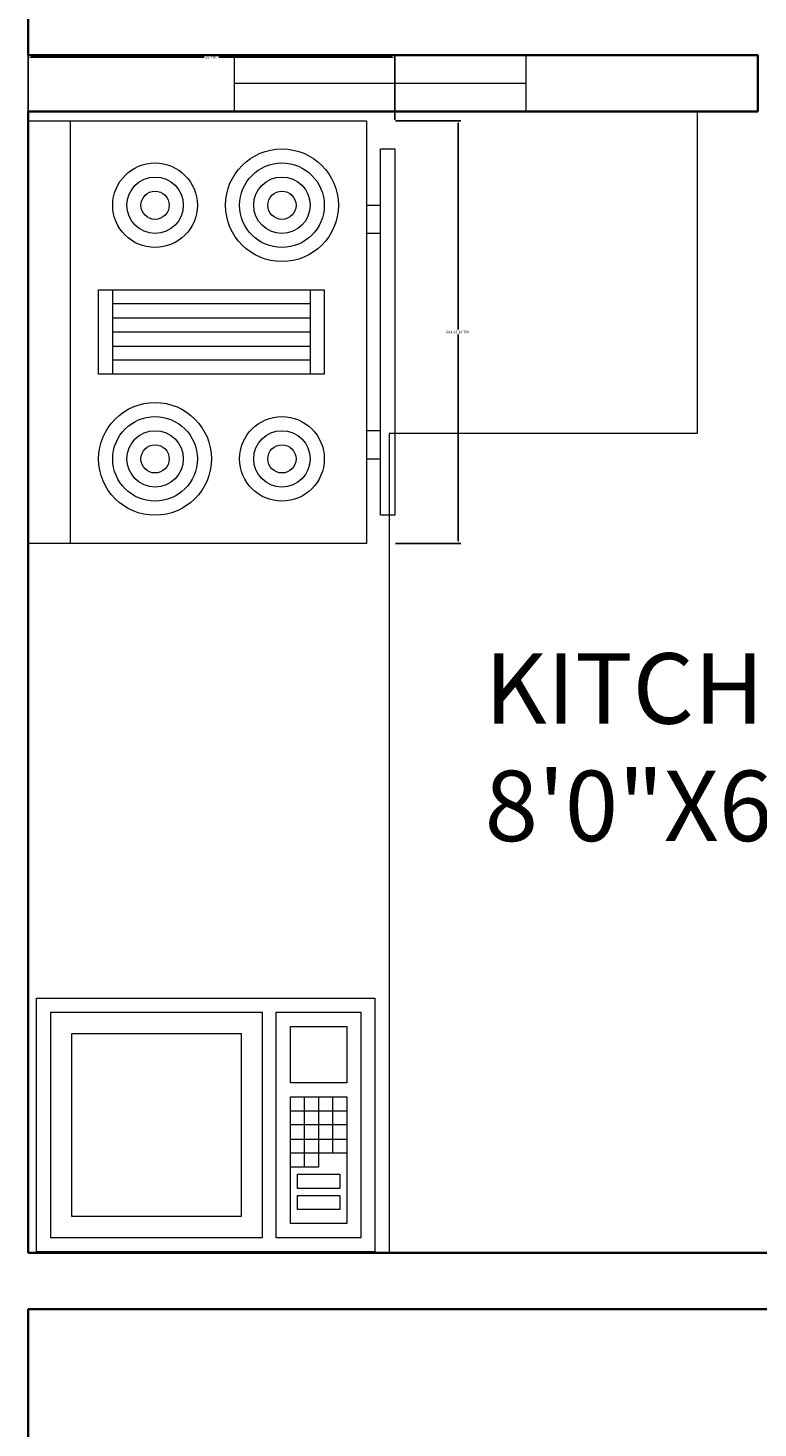
# Model space of a CAD drawing. Units: inches. Extents: x -86 to 2463, y -1058 to 68.
# Tile 13 of 17: x 25 to 77, y -114 to -14. Entities that reach past the tile are written whole.
import ezdxf

# ---------------------------------------------------------------- set-up
doc = ezdxf.new("R2010")
doc.units = ezdxf.units.IN
doc.header["$MEASUREMENT"] = 0
for name, color, linetype, lineweight in [('A-ANNO-DIMS', 2, 'Continuous', 18), ('A-AREA-IDEN', 7, 'Continuous', 18), ('A-EQPM', 9, 'Continuous', 18), ('A-FLOR-CASE', 8, 'Continuous', 18), ('A-GLAZ', 4, 'Continuous', 18), ('A-WALL', 7, 'Continuous', 35)]:
    doc.layers.add(name, color=color, linetype=linetype, lineweight=lineweight)
doc.styles.get("Standard").update_dxf_attribs({"font": 'arial.ttf'})
doc.dimstyles.get("Standard").update_dxf_attribs({"dimtxt": 0.18, "dimasz": 0.18, "dimexe": 0.18, "dimexo": 0.0625, "dimgap": 0.09, "dimtad": 0, "dimtih": 1, "dimtoh": 1, "dimdec": 4, "dimzin": 0, "dimdsep": 46, "dimtxsty": 'Standard', "dimcen": 0.09, "dimadec": 0, "dimazin": 0, "dimtfac": 1, "dimtdec": 4, "dimtofl": 0, "dimtmove": 0, "dimatfit": 3, "dimfxl": 1, "dimtolj": 1, "dimtzin": 0, "dimarcsym": 0})

# ---------------------------------------------------------------- blocks, each defined once
blk = doc.blocks.new('Microwave')
for p, q in [((19, 7), (19, 11)), ((20, 11), (20, 7)), ((21, 7), (21, 11)), ((18, 10), (22, 10)), ((22, 9), (18, 9)), ((18, 8), (22, 8)), ((22, 7), (18, 7)), ((19, 6), (19, 7)), ((20, 7), (20, 6)), ((20, 6), (18, 6))]:
    blk.add_line(p, q)
for points in [[(0, 0), (0, 18), (24, 18), (24, 0)], [(1, 1), (1, 17), (16, 17), (16, 1)], [(17, 1), (17, 17), (23, 17), (23, 1)], [(18, 12), (18, 16), (22, 16), (22, 12)], [(2.5, 2.5), (2.5, 15.5), (14.5, 15.5), (14.5, 2.5)], [(18, 2), (18, 11), (22, 11), (22, 2)], [(18.5, 4.5), (18.5, 5.5), (21.5, 5.5), (21.5, 4.5)], [(18.5, 3), (18.5, 4), (21.5, 4), (21.5, 3)]]:
    blk.add_lwpolyline(points, close=True)
blk = doc.blocks.new('Range-Oven - 30 in top')
for p, q in [((0, -3), (30, -3)), ((12, -6), (18, -6)), ((13, -20), (13, -6)), ((14, -6), (14, -20)), ((15, -20), (15, -6)), ((16, -6), (16, -20)), ((17, -20), (17, -6)), ((18, -20), (12, -20)), ((6, -24), (6, -25)), ((8, -25), (8, -24)), ((22, -25), (22, -24)), ((24, -24), (24, -25))]:
    blk.add_line(p, q)
for points in [[(0, -24), (0, 0), (30, 0), (30, -24)], [(12, -21), (12, -5), (18, -5), (18, -21)], [(2, -26), (2, -25), (28, -25), (28, -26)]]:
    blk.add_lwpolyline(points, close=True)
for centre, radius in [((6, -9), 4), ((6, -9), 3), ((24, -9), 3), ((6, -9), 2), ((24, -9), 2), ((6, -9), 1), ((24, -9), 1), ((24, -18), 4), ((6, -18), 3), ((24, -18), 3), ((6, -18), 2), ((24, -18), 2), ((6, -18), 1), ((24, -18), 1)]:
    blk.add_circle(centre, radius)
blk = doc.blocks.new('*D16')
at = {"layer": 'A-ANNO-DIMS', "color": 0, "lineweight": -2, "transparency": 16777216}
for p, q in [((50.834, -20.762), (55.451, -20.762)), ((55.271, -20.942), (55.271, -35.579)), ((55.271, -50.582), (55.271, -35.946)), ((50.834, -50.762), (55.451, -50.762))]:
    blk.add_line(p, q, dxfattribs=at)
at = {"layer": 'A-ANNO-DIMS', "color": 0, "transparency": 16777216}
for points in [[(55.241, -20.942), (55.301, -20.942), (55.271, -20.762)], [(55.241, -50.582), (55.301, -50.582), (55.271, -50.762)]]:
    blk.add_solid(points, dxfattribs=at)
at = {"layer": 'Defpoints', "color": 0, "transparency": 16777216}
for p in [(50.771, -20.762), (55.271, -20.762), (50.771, -50.762)]:
    blk.add_point(p, dxfattribs=at)
at = {"layer": 'A-ANNO-DIMS', "color": 0, "transparency": 16777216, "insert": (55.271, -35.762), "char_height": 0.18, "attachment_point": 5}
blk.add_mtext('\\A1;RANGE 30 TYP.', dxfattribs=at)
blk = doc.blocks.new('*D17')
at = {"layer": 'A-ANNO-DIMS', "color": 0, "lineweight": -2, "transparency": 16777216}
for p, q in [((24.771, -20.7), (24.771, -16.082)), ((24.951, -16.262), (37.242, -16.262)), ((50.591, -16.262), (38.301, -16.262)), ((50.771, -20.7), (50.771, -16.082))]:
    blk.add_line(p, q, dxfattribs=at)
at = {"layer": 'A-ANNO-DIMS', "color": 0, "transparency": 16777216}
for points in [[(24.951, -16.232), (24.951, -16.292), (24.771, -16.262)], [(50.591, -16.232), (50.591, -16.292), (50.771, -16.262)]]:
    blk.add_solid(points, dxfattribs=at)
at = {"layer": 'Defpoints', "color": 0, "transparency": 16777216}
for p in [(24.771, -16.262), (24.771, -20.762), (50.771, -20.762)]:
    blk.add_point(p, dxfattribs=at)
at = {"layer": 'A-ANNO-DIMS', "color": 0, "transparency": 16777216, "insert": (37.771, -16.262), "char_height": 0.18, "attachment_point": 5}
blk.add_mtext('\\A1;26 TYP.', dxfattribs=at)

msp = doc.modelspace()

# ---------------------------------------------------------------- linework, layer by layer
at = {"layer": 'A-FLOR-CASE'}
for p, q in [((72.212, -20.104), (72.212, -42.96)), ((72.212, -42.96), (50.384, -42.96)), ((50.384, -42.96), (50.384, -101.104))]:
    msp.add_line(p, q, dxfattribs=at)
at = {"layer": 'A-GLAZ'}
for p, q in [((39.392, -16.104), (39.392, -20.104)), ((60.06, -16.104), (60.06, -20.104)), ((39.392, -18.104), (60.06, -18.104))]:
    msp.add_line(p, q, dxfattribs=at)
at = {"layer": 'A-WALL'}
for p, q in [((24.761, -16.104), (24.761, 19.896)), ((76.532, -16.104), (24.761, -16.104)), ((76.532, -16.104), (76.532, -20.104)), ((24.761, -20.104), (24.761, -101.104)), ((76.532, -20.104), (24.761, -20.104)), ((106.761, -101.104), (24.761, -101.104)), ((102.761, -105.104), (24.761, -105.104)), ((24.761, -105.104), (24.761, -141.104))]:
    msp.add_line(p, q, dxfattribs=at)

# ---------------------------------------------------------------- block references
at = {"layer": 'A-EQPM', "rotation": 90}
msp.add_blockref('Range-Oven - 30 in top', (24.771, -50.762), dxfattribs=at)
at = {"layer": 'A-EQPM'}
msp.add_blockref('Microwave', (25.369, -101.04), dxfattribs=at)

# ---------------------------------------------------------------- texts
at = {"layer": 'A-AREA-IDEN', "insert": (57.148, -58.557), "char_height": 5, "attachment_point": 1}
msp.add_mtext_dynamic_manual_height_columns('KITCHEN\\P8\'0"X6\'9"', width=26.29818, gutter_width=25, heights=[0], dxfattribs=at)

# ---------------------------------------------------------------- dimensions: what is measured, and where the dimension line sits
at = {"layer": 'A-ANNO-DIMS'}
for base, p1, p2, angle, text, picture, middle in [((24.771, -16.262), (50.771, -20.762), (24.771, -20.762), 180, '<> TYP.', '*D17', (37.771, -16.262)), ((55.271, -20.762), (50.771, -50.762), (50.771, -20.762), 90, 'RANGE <> TYP.', '*D16', (55.271, -35.762))]:
    dim = msp.add_linear_dim(base=base, p1=p1, p2=p2, angle=angle, text=text, dimstyle='Standard', override={"dimdec": 0, "dimlfac": 1, "dimrnd": 0, "dimzin": 0, "dimdsep": 46, "dimlunit": 2}, dxfattribs=at)
    dim.commit()
    dim.dimension.update_dxf_attribs({"geometry": picture, "text_midpoint": middle})

doc.saveas('drawing.dxf')
